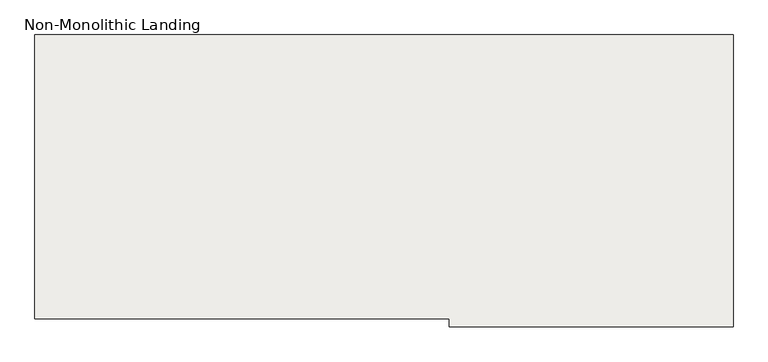
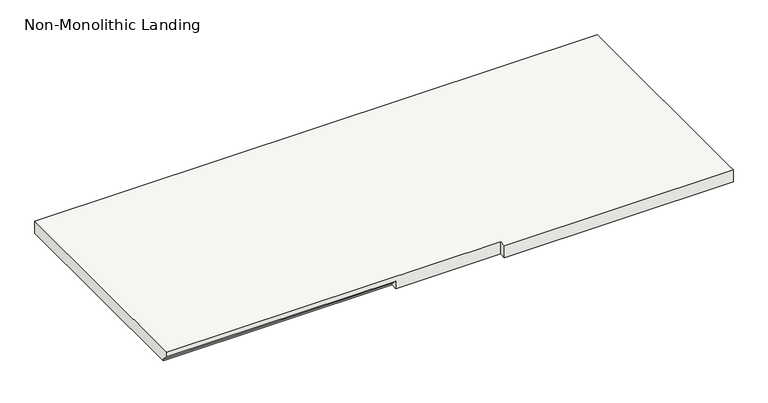
"""IFC4 building model written with IfcOpenShell, lengths in millimetres: slab geometry, Non-Monolithic Landing."""

from ifc_helpers import new_model, si_unit, origin, place, context, project, spatial, faceted_brep, source, transform, mapped, element, save


def non_monolithic_landing_99b9b51a(model_context):
    return source(origin(), model_context, "Body", "Brep", [
        faceted_brep([(131.9501403, 2113.4257925, 8413.75), (131.9501403, 2138.8257925, 8388.35), (1046.3501403, 2138.8257925, 8388.35), (1046.3501403, 2113.4257925, 8413.75), (1465.4501403, 2113.4257925, 8432.8), (1465.4501403, 2088.0257925, 8432.8), (2379.8501403, 2088.0257925, 8432.8), (2379.8501403, 2113.4257925, 8432.8), (2379.8501403, 3027.8257925, 8432.8), (131.9501403, 3027.8257925, 8432.8), (131.9501403, 2113.4257925, 8432.8), (1046.3501403, 2138.8257925, 8382.0), (131.9501403, 2138.8257925, 8382.0), (131.9501403, 3027.8257925, 8382.0), (2379.8501403, 3027.8257925, 8382.0), (2379.8501403, 2113.4257925, 8382.0), (2379.8501403, 2088.0257925, 8382.0), (1465.4501403, 2088.0257925, 8382.0), (1465.4501403, 2113.4257925, 8382.0), (1046.3501403, 2113.4257925, 8382.0)], [[[0, 1, 2, 3]], [[4, 5, 6, 7, 8, 9, 10]], [[11, 12, 13, 14, 15, 16, 17, 18, 19]], [[12, 11, 2, 1]], [[11, 19, 3, 2]], [[4, 10, 0, 3, 19, 18]], [[5, 4, 18, 17]], [[6, 5, 17, 16]], [[7, 6, 16, 15]], [[8, 7, 15, 14]], [[9, 8, 14, 13]], [[10, 9, 13, 12, 1, 0]]]),
    ])


if __name__ == "__main__":
    model = new_model("IFC4")
    model_context = context("Model", 3, world=origin())
    ifc_project = project(units=[si_unit("LENGTHUNIT", "METRE", prefix="MILLI")], contexts=[model_context])
    site = spatial("IfcSite", under=ifc_project)
    building = spatial("IfcBuilding", under=site)
    placement = place(None, origin())
    non_monolithic_landing_shape = non_monolithic_landing_99b9b51a(model_context)
    element("IfcSlab", 1, ObjectType="Non-Monolithic Landing", at=placement, inside=building, context=model_context, shape_type="MappedRepresentation", body=[
        mapped(non_monolithic_landing_shape, transform((0.0, 0.0, 0.0), x_axis=(1.0, 0.0, 0.0), y_axis=(0.0, 1.0, 0.0), z_axis=(0.0, 0.0, 1.0))),
    ])
    save(model, "model.ifc")
